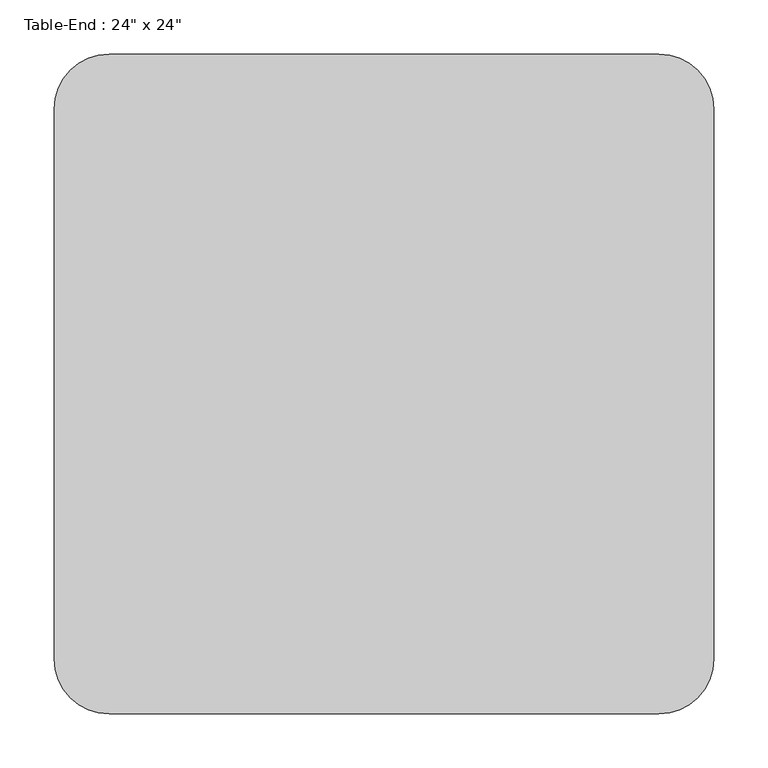
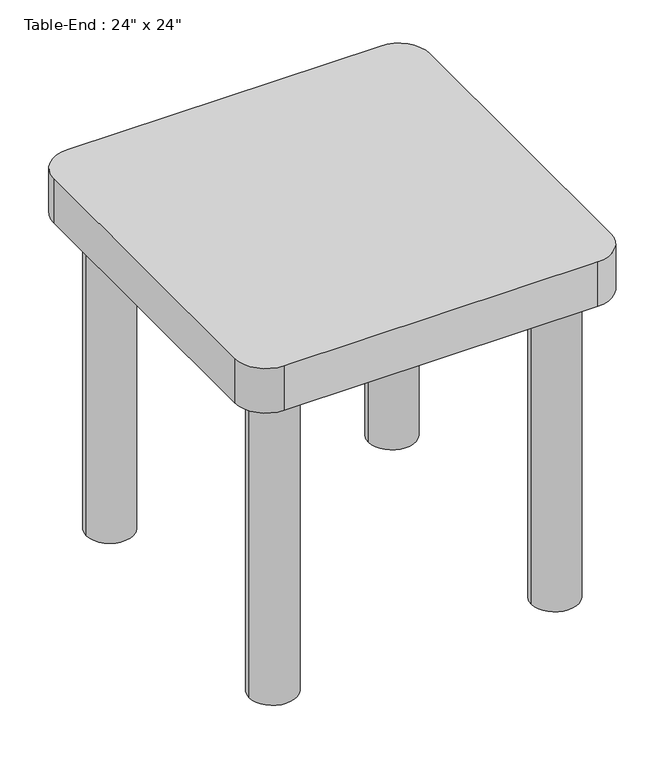
"""IFC4 building model written with IfcOpenShell, lengths in millimetres: furniture geometry."""

from ifc_helpers import new_model, si_unit, point, frame, frame_2d, origin, origin_with_axes, place, context, project, spatial, polyline, circle_curve, trimmed, segment, composite_curve, outline, extrude, source, transform, mapped, element, save


def furniture_31d08a24(model_context):
    return source(origin(), model_context, "Body", "SweptSolid", [
        extrude(outline(composite_curve([segment(polyline([(562.5336303, -152.4), (54.5336303, -152.4)]), True, "CONTINUOUS"), segment(trimmed(circle_curve(frame_2d((54.5336303, -101.6)), 50.8), [point((54.5336303, -152.4))], [point((3.7336303, -101.6))], False, "CARTESIAN"), True, "CONTINUOUS"), segment(polyline([(3.7336303, -101.6), (3.7336303, 406.4)]), True, "CONTINUOUS"), segment(trimmed(circle_curve(frame_2d((54.5336303, 406.4)), 50.8), [point((3.7336303, 406.4))], [point((54.5336303, 457.2))], False, "CARTESIAN"), True, "CONTINUOUS"), segment(polyline([(54.5336303, 457.2), (562.5336303, 457.2)]), True, "CONTINUOUS"), segment(trimmed(circle_curve(frame_2d((562.5336303, 406.4)), 50.8), [point((562.5336303, 457.2))], [point((613.3336303, 406.4))], False, "CARTESIAN"), True, "CONTINUOUS"), segment(polyline([(613.3336303, 406.4), (613.3336303, -101.6)]), True, "CONTINUOUS"), segment(trimmed(circle_curve(frame_2d((562.5336303, -101.6)), 50.8), [point((613.3336303, -101.6))], [point((562.5336303, -152.4))], False, "CARTESIAN"), True, "CONTINUOUS")], self_intersect=False)), frame((0.0, 0.0, 533.4), z_axis=(0.0, 0.0, 1.0), x_axis=(1.0, 0.0, 0.0)), (0.0, 0.0, 1.0), 76.2),
        extrude(outline(composite_curve([segment(trimmed(circle_curve(frame_2d((79.9336303, 381.0)), 38.1), [point((41.8336303, 381.0))], [point((118.0336303, 381.0))], False, "CARTESIAN"), True, "CONTINUOUS"), segment(trimmed(circle_curve(frame_2d((79.9336303, 381.0)), 38.1), [point((118.0336303, 381.0))], [point((41.8336303, 381.0))], False, "CARTESIAN"), True, "CONTINUOUS")], self_intersect=False)), origin_with_axes(), (0.0, 0.0, 1.0), 533.4),
        extrude(outline(composite_curve([segment(trimmed(circle_curve(frame_2d((79.9336303, -76.2)), 38.1), [point((41.8336303, -76.2))], [point((118.0336303, -76.2))], False, "CARTESIAN"), True, "CONTINUOUS"), segment(trimmed(circle_curve(frame_2d((79.9336303, -76.2)), 38.1), [point((118.0336303, -76.2))], [point((41.8336303, -76.2))], False, "CARTESIAN"), True, "CONTINUOUS")], self_intersect=False)), origin_with_axes(), (0.0, 0.0, 1.0), 533.4),
        extrude(outline(composite_curve([segment(trimmed(circle_curve(frame_2d((537.1336303, -76.2)), 38.1), [point((499.0336303, -76.2))], [point((575.2336303, -76.2))], False, "CARTESIAN"), True, "CONTINUOUS"), segment(trimmed(circle_curve(frame_2d((537.1336303, -76.2)), 38.1), [point((575.2336303, -76.2))], [point((499.0336303, -76.2))], False, "CARTESIAN"), True, "CONTINUOUS")], self_intersect=False)), origin_with_axes(), (0.0, 0.0, 1.0), 533.4),
        extrude(outline(composite_curve([segment(trimmed(circle_curve(frame_2d((537.1336303, 381.0)), 38.1), [point((499.0336303, 381.0))], [point((575.2336303, 381.0))], False, "CARTESIAN"), True, "CONTINUOUS"), segment(trimmed(circle_curve(frame_2d((537.1336303, 381.0)), 38.1), [point((575.2336303, 381.0))], [point((499.0336303, 381.0))], False, "CARTESIAN"), True, "CONTINUOUS")], self_intersect=False)), origin_with_axes(), (0.0, 0.0, 1.0), 533.4),
    ])


if __name__ == "__main__":
    model = new_model("IFC4")
    model_context = context("Model", 3, world=origin())
    ifc_project = project(units=[si_unit("LENGTHUNIT", "METRE", prefix="MILLI")], contexts=[model_context])
    site = spatial("IfcSite", under=ifc_project)
    building = spatial("IfcBuilding", under=site)
    placement = place(None, origin())
    furniture_shape = furniture_31d08a24(model_context)
    element("IfcFurniture", 1, ObjectType="Table-End : 24\" x 24\"", at=placement, inside=building, context=model_context, shape_type="MappedRepresentation", body=[
        mapped(furniture_shape, transform((0.0, 0.0, 0.0), x_axis=(1.0, 0.0, 0.0), y_axis=(0.0, 1.0, 0.0), z_axis=(0.0, 0.0, 1.0))),
    ])
    save(model, "model.ifc")

# Revit data of these elements
# Type "Table-End : 24\" x 24\""
#   Assembly Code = "E2020200"
#   Height = 2' - 0"
#   Length = 2' - 0"
#   Width = 2' - 0"
#   Base Material = Birch
#   Top Material = Laminate, Ivory, Matte
#   Default Elevation = 0
# Element 1 (IfcFurniture, "Table-End : 24\" x 24\"")
#   Materials on its faces: "Laminate, Ivory, Matte", "Birch"
# Materials
#   "Birch": class "Wood", colour RGB 224 178 126, transparency 0, Description = "Betula Alleghaniensis", Cost = 0
#   "Laminate, Ivory, Matte": class "Plastic", colour RGB 247 247 239, transparency 0, Description = "Plastic Laminate - Ivory, Matte", Cost = 0
